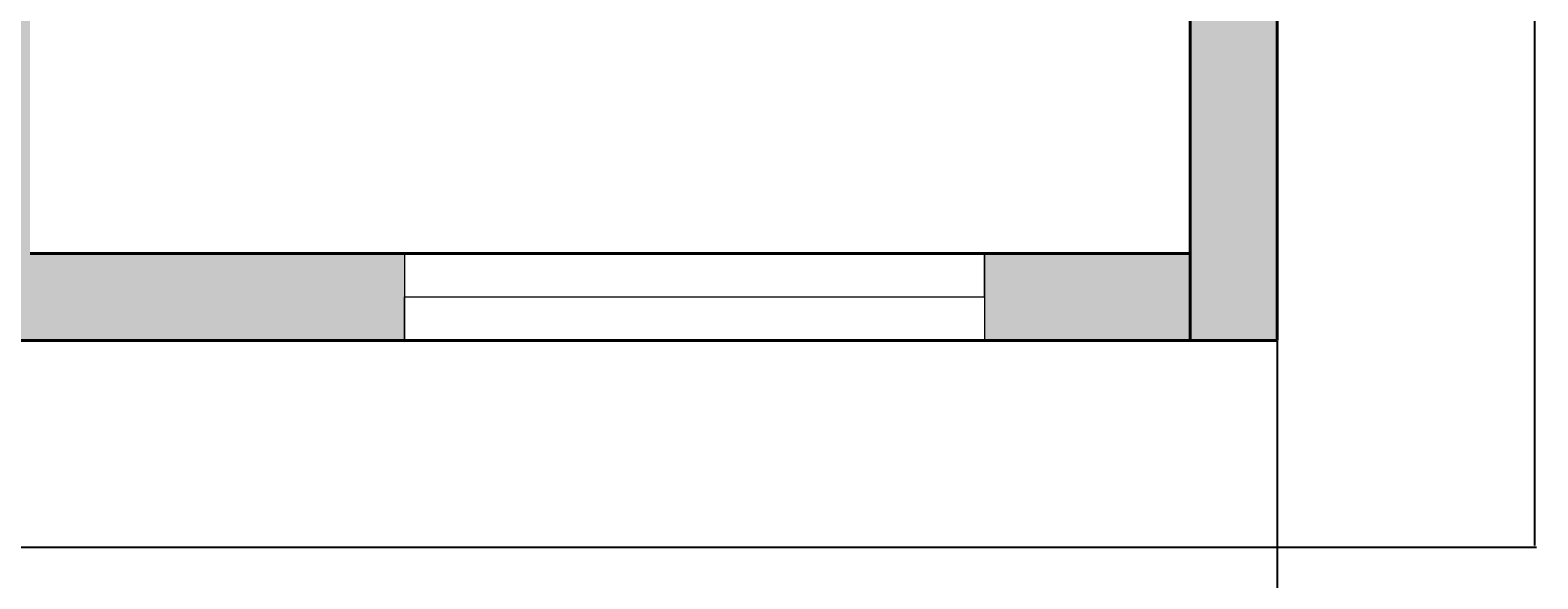
# Model space of a CAD drawing. Units: inches. Extents: x 1441 to 2460, y 1648 to 2683.
# Tile 3 of 35: x 1760 to 1916, y 1810 to 1866. Entities that reach past the tile are written whole.
import ezdxf

# ---------------------------------------------------------------- set-up
doc = ezdxf.new("R2010")
doc.units = ezdxf.units.IN
for name, color, linetype, lineweight in [('A-ANNO-DIMS', 2, 'Continuous', 18), ('A-GLAZ', 4, 'Continuous', 18), ('A-WALL', 7, 'Continuous', 40)]:
    doc.layers.add(name, color=color, linetype=linetype, lineweight=lineweight)
doc.layers.add('A-WALL-PATT', color=251, linetype='Continuous', lineweight=13, true_color=0x636466)
doc.styles.get("Standard").update_dxf_attribs({"font": 'arial.ttf'})
doc.dimstyles.get("Standard").update_dxf_attribs({"dimtxt": 0.18, "dimasz": 0.18, "dimexe": 0.18, "dimexo": 0.0625, "dimgap": 0.09, "dimtad": 0, "dimtih": 1, "dimtoh": 1, "dimdec": 4, "dimzin": 0, "dimdsep": 46, "dimtxsty": 'Standard', "dimcen": 0.09, "dimadec": 0, "dimazin": 0, "dimtfac": 1, "dimtdec": 4, "dimtofl": 0, "dimtmove": 0, "dimatfit": 3, "dimfxl": 1, "dimtolj": 1, "dimtzin": 0, "dimarcsym": 0})

# ---------------------------------------------------------------- blocks, each defined once
blk = doc.blocks.new('*D66')
at = {"layer": 'A-ANNO-DIMS', "color": 0, "lineweight": -2, "transparency": 16777216}
for p, q in [((1568.89, 1834.13), (1568.89, 1745.01)), ((1889.39, 1834.13), (1889.39, 1745.01)), ((1569.07, 1745.19), (1728.74, 1745.19)), ((1889.21, 1745.19), (1729.53, 1745.19))]:
    blk.add_line(p, q, dxfattribs=at)
at = {"layer": 'A-ANNO-DIMS', "color": 0, "transparency": 16777216}
for points in [[(1569.07, 1745.22), (1569.07, 1745.16), (1568.89, 1745.19)], [(1889.21, 1745.22), (1889.21, 1745.16), (1889.39, 1745.19)]]:
    blk.add_solid(points, dxfattribs=at)
at = {"layer": 'Defpoints', "color": 0, "transparency": 16777216}
for p in [(1568.89, 1834.2), (1889.39, 1834.2), (1889.39, 1745.19)]:
    blk.add_point(p, dxfattribs=at)
at = {"layer": 'A-ANNO-DIMS', "color": 0, "transparency": 16777216, "insert": (1729.14, 1745.19), "char_height": 0.18, "attachment_point": 5}
blk.add_mtext('\\A1;320.5', dxfattribs=at)
blk = doc.blocks.new('*D67')
at = {"layer": 'A-ANNO-DIMS', "color": 0, "lineweight": -2, "transparency": 16777216}
for p, q in [((1889.45, 2298.7), (1916.22, 2298.7)), ((1916.04, 2298.52), (1916.04, 2055.94)), ((1916.04, 1813), (1916.04, 2055.57)), ((1758.22, 1812.82), (1916.22, 1812.82))]:
    blk.add_line(p, q, dxfattribs=at)
at = {"layer": 'A-ANNO-DIMS', "color": 0, "transparency": 16777216}
for points in [[(1916.01, 2298.52), (1916.07, 2298.52), (1916.04, 2298.7)], [(1916.01, 1813), (1916.07, 1813), (1916.04, 1812.82)]]:
    blk.add_solid(points, dxfattribs=at)
at = {"layer": 'Defpoints', "color": 0, "transparency": 16777216}
for p in [(1889.39, 2298.7), (1916.04, 2298.7), (1758.16, 1812.82)]:
    blk.add_point(p, dxfattribs=at)
at = {"layer": 'A-ANNO-DIMS', "color": 0, "transparency": 16777216, "insert": (1916.04, 2055.76), "char_height": 0.18, "attachment_point": 5}
blk.add_mtext('\\A1;485.9', dxfattribs=at)

msp = doc.modelspace()

# ---------------------------------------------------------------- hatches: boundary and pattern name
at = {"layer": 'A-WALL-PATT'}
h = msp.add_hatch(color=256, dxfattribs=at)
h.dxf.hatch_style = 1
h.paths.add_polyline_path([(1627.5085, 2298.6952), (1568.8859, 2298.6952), (1568.8859, 2246.9605), (1577.8859, 2246.9605), (1577.8859, 2289.6952), (1627.5085, 2289.6952), (1627.5085, 2294.1952)])
h.paths.add_polyline_path([(1675.5777, 2298.6952), (1651.5085, 2298.6952), (1651.5085, 2289.6952), (1675.5777, 2289.6952), (1675.5777, 2294.1952)])
h.paths.add_polyline_path([(1667.3859, 2289.6952), (1662.8859, 2289.6952), (1662.8859, 2233.0622), (1667.3859, 2233.0622)])
h.paths.add_polyline_path([(1715.8721, 2294.3362), (1715.8721, 2295.2788), (1715.8721, 2298.6952), (1699.5777, 2298.6952), (1699.5777, 2289.6952), (1715.8721, 2289.6952)])
h.paths.add_polyline_path([(1707.8859, 2289.6952), (1703.3859, 2289.6952), (1703.3859, 2199.6952), (1707.8859, 2199.6952)])
h.paths.add_polyline_path([(1760.3859, 2204.637), (1755.8859, 2204.637), (1755.8859, 2199.6952), (1667.3859, 2199.6952), (1667.3859, 2204.637), (1662.8859, 2204.637), (1662.8859, 2195.1952), (1760.3859, 2195.1952)])
h.paths.add_polyline_path([(1760.3859, 2289.6952), (1755.8859, 2289.6952), (1755.8859, 2233.0622), (1760.3859, 2233.0622)])
h.paths.add_polyline_path([(1889.3859, 2298.6952), (1739.8721, 2298.6952), (1739.8721, 2289.6952), (1880.3859, 2289.6952), (1880.3859, 2250.8051), (1889.3859, 2250.8051)])
h.paths.add_polyline_path([(1889.3859, 2202.8051), (1880.3859, 2202.8051), (1880.3859, 2157.6952), (1747.948, 2157.6952), (1747.948, 2153.1952), (1755.8859, 2153.1952), (1755.8859, 2058.005), (1760.3859, 2058.005), (1760.3859, 2153.1952), (1880.3859, 2153.1952), (1880.3859, 2124.108), (1889.3859, 2124.108)])
h.paths.add_polyline_path([(1889.3859, 1984.8305), (1880.3859, 1984.8305), (1880.3859, 1834.1952), (1889.3859, 1834.1952)])
h.paths.add_polyline_path([(1889.3859, 2076.108), (1880.3859, 2076.108), (1880.3859, 2008.8305), (1889.3859, 2008.8305)])
h.paths.add_polyline_path([(1880.3859, 2027.1952), (1800.8859, 2027.1952), (1800.8859, 2000.9452), (1805.3859, 2000.9452), (1805.3859, 2022.6952), (1880.3859, 2022.6952)])
h.paths.add_polyline_path([(1800.8859, 2027.1952), (1760.3859, 2027.1952), (1760.3859, 2030.7912), (1755.8859, 2030.7912), (1755.8859, 2022.6952), (1800.8859, 2022.6952)])
h.paths.add_polyline_path([(1880.3859, 1974.6952), (1805.3859, 1974.6952), (1805.3859, 1978.7973), (1800.8859, 1978.7973), (1800.8859, 1974.6952), (1794.8823, 1974.6952), (1794.8823, 1970.1952), (1800.8859, 1970.1952), (1805.3859, 1970.1952), (1880.3859, 1970.1952)])
h.paths.add_polyline_path([(1760.3859, 1974.6952), (1755.8859, 1974.6952), (1755.8859, 1925.6952), (1751.8616, 1925.6952), (1751.8616, 1921.1952), (1760.3859, 1921.1952)])
h.paths.add_polyline_path([(1760.3859, 1921.1952), (1755.8859, 1921.1952), (1755.8859, 1843.1952), (1760.3859, 1843.1952)])
h.paths.add_polyline_path([(1799.1136, 1838.6952), (1799.1136, 1843.1952), (1760.3859, 1843.1952), (1751.8944, 1843.1952), (1751.8944, 1834.1952), (1758.1615, 1834.1952), (1799.1136, 1834.1952)])
h.paths.add_polyline_path([(1880.3859, 1843.1952), (1859.1136, 1843.1952), (1859.1136, 1834.1952), (1880.3859, 1834.1952)])
h.paths.add_polyline_path([(1577.8859, 1857.7914), (1568.8859, 1857.7914), (1568.8859, 1834.1952), (1695.0034, 1834.1952), (1695.0034, 1838.6952), (1695.0034, 1843.1952), (1577.8859, 1843.1952)])
h.paths.add_polyline_path([(1577.8859, 1959.2399), (1573.3859, 1959.2399), (1568.8859, 1959.2399), (1568.8859, 1905.7914), (1577.8859, 1905.7914), (1577.8859, 1921.1952), (1703.3859, 1921.1952), (1707.8859, 1921.1952), (1715.1501, 1921.1952), (1715.1501, 1925.6952), (1707.8859, 1925.6952), (1703.3859, 1925.6952), (1577.8859, 1925.6952)])
h.paths.add_polyline_path([(1577.8859, 2106.6907), (1568.8859, 2106.6907), (1568.8859, 2019.2399), (1577.8859, 2019.2399)])
h.paths.add_polyline_path([(1707.8859, 2051.6952), (1703.3859, 2051.6952), (1703.3859, 2048.6952), (1703.3859, 1925.6952), (1707.8859, 1925.6952)])
h.paths.add_polyline_path([(1703.3859, 2051.6952), (1676.3859, 2051.6952), (1676.3859, 2048.6952), (1703.3859, 2048.6952)])
h.paths.add_polyline_path([(1703.3859, 2102.6952), (1676.3859, 2102.6952), (1676.3859, 2099.6952), (1685.3859, 2099.6952), (1703.3859, 2099.6952)])
h.paths.add_polyline_path([(1707.8859, 2153.1952), (1710.5611, 2153.1952), (1710.5611, 2157.6952), (1707.8859, 2157.6952), (1707.8859, 2195.1952), (1703.3859, 2195.1952), (1703.3859, 2099.6952), (1707.8859, 2099.6952)])
h.paths.add_polyline_path([(1577.8859, 2198.9605), (1568.8859, 2198.9605), (1568.8859, 2166.6907), (1577.8859, 2166.6907)])

# ---------------------------------------------------------------- linework, layer by layer
at = {"layer": 'A-GLAZ'}
for p, q in [((1799.1136, 1843.1952), (1799.1136, 1834.1952)), ((1859.1136, 1838.6952), (1859.1136, 1843.1952)), ((1859.1136, 1843.1952), (1859.1136, 1834.1952)), ((1799.1136, 1834.1952), (1799.1136, 1838.6952)), ((1799.1136, 1838.6952), (1799.1136, 1838.6952)), ((1799.1136, 1838.6952), (1859.1136, 1838.6952))]:
    msp.add_line(p, q, dxfattribs=at)
at = {"layer": 'A-WALL'}
for p, q in [((1889.3859, 2298.6952), (1889.3859, 1834.1952)), ((1880.3859, 2153.1952), (1880.3859, 1834.1952)), ((1760.3859, 1843.1952), (1880.3859, 1843.1952)), ((1751.8944, 1834.1952), (1880.3859, 1834.1952)), ((1880.3859, 1834.1952), (1889.3859, 1834.1952))]:
    msp.add_line(p, q, dxfattribs=at)

# ---------------------------------------------------------------- dimensions: what is measured, and where the dimension line sits
at = {"layer": 'A-ANNO-DIMS'}
dim = msp.add_linear_dim(base=(1916.0359, 2298.6952), p1=(1758.1615, 1812.8171), p2=(1889.3859, 2298.6952), angle=90, dimstyle='Standard', override={"dimdec": 1, "dimlfac": 1, "dimrnd": 0, "dimzin": 0, "dimdsep": 46, "dimlunit": 2}, dxfattribs=at)
dim.commit()
dim.dimension.update_dxf_attribs({"geometry": '*D67', "text_midpoint": (1916.0359, 2055.7561)})
dim = msp.add_linear_dim(base=(1889.3859, 1745.1864), p1=(1568.8859, 1834.1952), p2=(1889.3859, 1834.1952), dimstyle='Standard', override={"dimdec": 1, "dimlfac": 1, "dimrnd": 0, "dimzin": 0, "dimdsep": 46, "dimlunit": 2}, dxfattribs=at)
dim.commit()
dim.dimension.update_dxf_attribs({"geometry": '*D66', "text_midpoint": (1729.1359, 1745.1864)})

doc.saveas('drawing.dxf')
